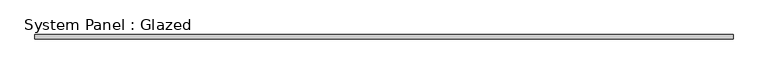
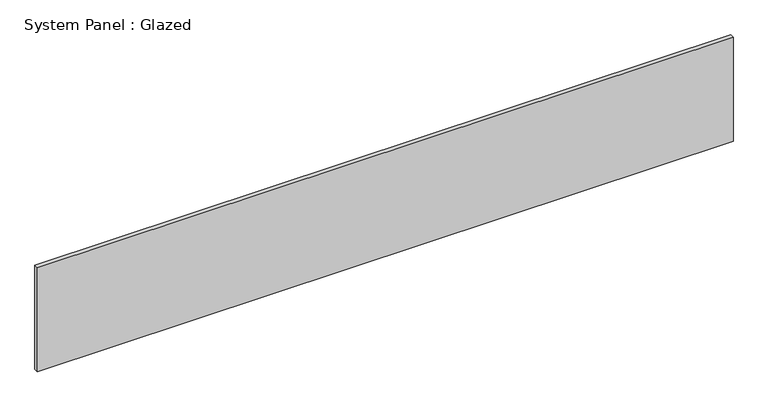
"""IFC4 building model written with IfcOpenShell, lengths in millimetres: plate geometry, System Panel : Glazed."""

from ifc_helpers import new_model, si_unit, origin, origin_with_axes, place, context, project, spatial, polyline, outline, extrude, source, transform, mapped, element, save


def system_panel_glazed_06e0175a(model_context):
    return source(origin(), model_context, "Body", "SweptSolid", [
        extrude(outline(polyline([(2095.5, 19.05), (-2095.5, 19.05), (-2095.5, 44.45), (2095.5, 44.45), (2095.5, 19.05)])), origin_with_axes(), (0.0, 0.0, 1.0), 662.2841344),
    ])


if __name__ == "__main__":
    model = new_model("IFC4")
    model_context = context("Model", 3, world=origin())
    ifc_project = project(units=[si_unit("LENGTHUNIT", "METRE", prefix="MILLI")], contexts=[model_context])
    site = spatial("IfcSite", under=ifc_project)
    building = spatial("IfcBuilding", under=site)
    placement = place(None, origin())
    system_panel_glazed_shape = system_panel_glazed_06e0175a(model_context)
    element("IfcPlate", 1, ObjectType="System Panel : Glazed", at=placement, inside=building, context=model_context, shape_type="MappedRepresentation", body=[
        mapped(system_panel_glazed_shape, transform((0.0, 0.0, 0.0), x_axis=(1.0, 0.0, 0.0), y_axis=(0.0, 1.0, 0.0), z_axis=(0.0, 0.0, 1.0))),
    ])
    save(model, "model.ifc")

# Revit data of these elements
# Type "System Panel : Glazed"
#   Construction Type Id = "GSP4R"
#   Analytic Construction = "1/8 in Pilkington single glazing"
#   Visual Light Transmittance = 0.9
#   Solar Heat Gain Coefficient = 0.86
#   Heat Transfer Coefficient (U) = 1.18115 BTU/(h·ft²·°F)
#   Define Thermal Properties by = 1
# Element 1 (IfcPlate, "System Panel : Glazed")
#   Materials on its faces: "Glass"
# Materials
#   "Glass": class "Glass", colour RGB 0 128 192, transparency 0.75, Description = "Soda Lime Glass", Cost = 0
